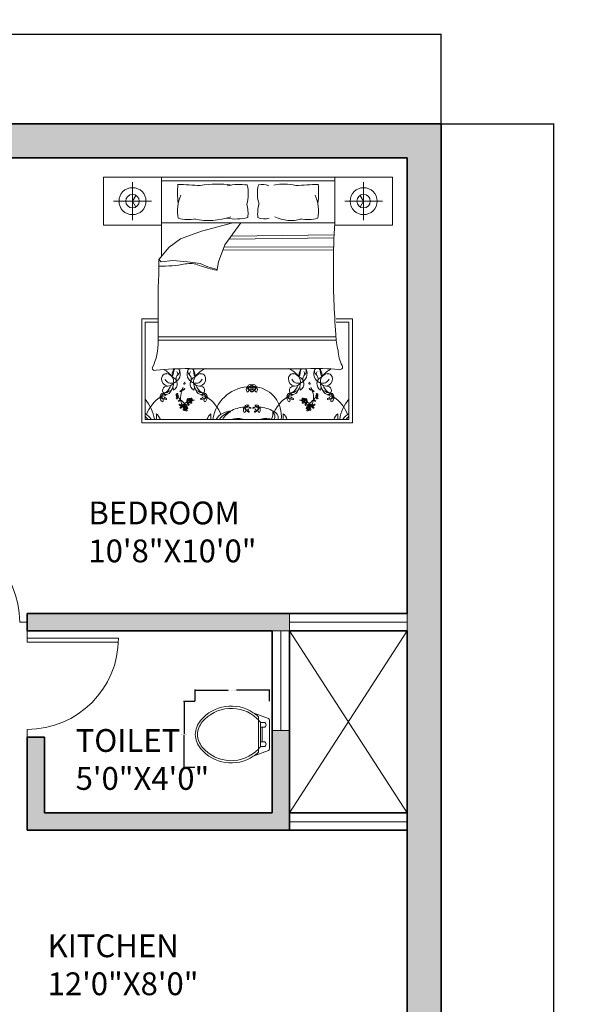
# Model space of a CAD drawing. Units: inches. Extents: x -5 to 366, y -496 to 54.
# Tile 10 of 10: x 214 to 366, y -205 to 54. Entities that reach past the tile are written whole.
import ezdxf

# ---------------------------------------------------------------- set-up
doc = ezdxf.new("R2010")
doc.units = ezdxf.units.IN
doc.header["$MEASUREMENT"] = 0
for name, color, linetype, lineweight in [('A-ANNO-DIMS', 2, 'Continuous', 18), ('A-AREA-IDEN', 7, 'Continuous', 25), ('A-DOOR', 3, 'Continuous', 18), ('A-FLOR-FIXT', 9, 'Continuous', 18), ('A-FLOR-OPEN', 8, 'Continuous', 13), ('A-FURN', 8, 'Continuous', 18), ('A-GLAZ', 4, 'Continuous', 18), ('A-WALL', 7, 'Continuous', 35), ('A-WALL-PATT', 252, 'Continuous', 13)]:
    doc.layers.add(name, color=color, linetype=linetype, lineweight=lineweight)
doc.styles.get("Standard").update_dxf_attribs({"font": 'arial.ttf'})
doc.dimstyles.get("Standard").update_dxf_attribs({"dimtxt": 0.18, "dimasz": 0.18, "dimexe": 0.18, "dimexo": 0.0625, "dimgap": 0.09, "dimtad": 0, "dimtih": 1, "dimtoh": 1, "dimdec": 0, "dimzin": 0, "dimdsep": 46, "dimlunit": 3, "dimtxsty": 'Standard', "dimcen": 0.09, "dimadec": 0, "dimazin": 0, "dimtfac": 1, "dimtdec": 0, "dimtofl": 0, "dimtmove": 0, "dimatfit": 3, "dimfxl": 1, "dimtolj": 1, "dimtzin": 0, "dimarcsym": 0})

# ---------------------------------------------------------------- blocks, each defined once
blk = doc.blocks.new('*D2')
at = {"layer": 'A-ANNO-DIMS', "color": 0, "lineweight": -2, "transparency": 16777216}
for p, q in [((21.93, 26.58), (21.93, 50.16)), ((22.11, 49.98), (162.99, 49.98)), ((324.75, 49.98), (183.88, 49.98)), ((324.93, 26.58), (324.93, 50.16))]:
    blk.add_line(p, q, dxfattribs=at)
at = {"layer": 'A-ANNO-DIMS', "color": 0, "transparency": 16777216}
for points in [[(22.11, 50.01), (22.11, 49.95), (21.93, 49.98)], [(324.75, 50.01), (324.75, 49.95), (324.93, 49.98)]]:
    blk.add_solid(points, dxfattribs=at)
at = {"layer": 'Defpoints', "color": 0, "transparency": 16777216}
for p in [(324.93, 49.98), (21.93, 26.52), (324.93, 26.52)]:
    blk.add_point(p, dxfattribs=at)
at = {"layer": 'A-ANNO-DIMS', "color": 0, "transparency": 16777216, "insert": (173.43, 49.98), "char_height": 6, "attachment_point": 5}
blk.add_mtext('\\A1;25\'-3"', dxfattribs=at)
blk = doc.blocks.new('*D3')
at = {"layer": 'A-ANNO-DIMS', "color": 0, "lineweight": -2, "transparency": 16777216}
for p, q in [((325, 26.52), (354.61, 26.52)), ((354.43, 26.34), (354.43, -212.08)), ((354.43, -456.8), (354.43, -218.38)), ((325, -456.98), (354.61, -456.98))]:
    blk.add_line(p, q, dxfattribs=at)
at = {"layer": 'A-ANNO-DIMS', "color": 0, "transparency": 16777216}
for points in [[(354.4, 26.34), (354.46, 26.34), (354.43, 26.52)], [(354.4, -456.8), (354.46, -456.8), (354.43, -456.98)]]:
    blk.add_solid(points, dxfattribs=at)
at = {"layer": 'Defpoints', "color": 0, "transparency": 16777216}
for p in [(324.93, 26.52), (324.93, -456.98), (354.43, -456.98)]:
    blk.add_point(p, dxfattribs=at)
at = {"layer": 'A-ANNO-DIMS', "color": 0, "transparency": 16777216, "insert": (354.43, -215.23), "char_height": 6, "attachment_point": 5}
blk.add_mtext('\\A1;40\'-4"', dxfattribs=at)
blk = doc.blocks.new('DOOR-SWING-24IN')
for p, q in [((-1, 0), (-1, 24)), ((0, 0), (0, 24))]:
    blk.add_line(p, q)
blk.add_arc((0, 0), 24, 90, 180)
blk = doc.blocks.new('BED-DOUBLE-WITH-NIGHTSTANDS')
for p, q in [((0, 64.67), (76.05, 64.67)), ((7.61, 53.37), (7.61, 63.31)), ((15.21, 64.67), (15.21, 43.8)), ((60.84, 63.7), (15.21, 63.7)), ((68.45, 53.37), (68.45, 63.31)), ((12.58, 58.34), (2.64, 58.34)), ((63.48, 58.34), (73.42, 58.34)), ((15.21, 52.66), (60.84, 52.66)), ((25.78, 50.4), (34.07, 52.66)), ((36.11, 52.66), (31.94, 46.86)), ((20.23, 48.39), (25.78, 50.4)), ((60.64, 49.5), (33.56, 49.12)), ((17.3, 46.24), (20.23, 48.39)), ((31.94, 46.86), (30.24, 42.39)), ((60.61, 48.72), (33, 48.33)), ((14.53, 43.01), (17.3, 46.24)), ((60.58, 45.54), (31.39, 45.42)), ((60.57, 46.32), (31.69, 46.21)), ((15.15, 42.39), (14.53, 43.01)), ((18.23, 42.7), (15.15, 42.39)), ((22.08, 42.39), (18.23, 42.7)), ((25.47, 41.93), (22.08, 42.39)), ((27.47, 41.01), (25.47, 41.93)), ((30.24, 42.39), (29.94, 40.39)), ((29.94, 40.39), (27.47, 41.01)), ((10.04, 27.39), (14.34, 27.39)), ((10.04, 0), (10.04, 27.39)), ((14.34, 26.51), (10.92, 26.51)), ((10.92, 26.51), (10.92, 0.88)), ((64.6, 26.51), (61.25, 26.51)), ((61.27, 27.39), (65.49, 27.39)), ((64.6, 0.88), (64.6, 26.51)), ((65.49, 27.39), (65.49, 0)), ((61.19, 22.65), (14.34, 22.65)), ((61.26, 21.7), (14.34, 21.7)), ((53.47, 14.23), (22.59, 14.23)), ((18.42, 8.59), (18.25, 9.45)), ((23.73, 8.59), (23.9, 9.45)), ((51.79, 8.59), (51.63, 9.45)), ((57.11, 8.59), (57.28, 9.45)), ((10.92, 0.88), (64.6, 0.88)), ((65.49, 0), (10.04, 0))]:
    blk.add_line(p, q)
for points in [[(15.21, 52), (0, 52), (0, 64.67)], [(60.84, 64.67), (60.84, 52), (76.05, 52), (76.05, 64.67)], [(7.61, 58.34), (8.49, 59.87)], [(68.45, 58.34), (67.56, 59.87)], [(7.61, 58.34), (8.49, 56.8)], [(68.45, 58.34), (67.56, 56.8)]]:
    blk.add_lwpolyline(points)
for points in [[(19.58, 62.78, 0.074897), (19.67, 57.81, -0.472817)], [(37.67, 57.53, 0.14099), (37.82, 62.6, 0.235245)], [(40.92, 57.53, -0.14099), (40.77, 62.6, -0.235245)], [(56.48, 62.78, -0.074897), (56.38, 57.81, 0.472817)], [(14.37, 36.04, 0.001242), (14.34, 21.61, -0.127202), (12.81, 14.42)], [(61.17, 23.25, 0.056112), (61.72, 19.07, 0.095341), (62.79, 15.03)]]:
    blk.add_lwpolyline(points, format="xyb")
for centre, radius in [((7.61, 58.34), 3.55), ((7.61, 58.34), 1.77), ((68.45, 58.34), 3.55), ((68.45, 58.34), 1.77), ((22.81, 5.83), 0.194), ((52.72, 5.83), 0.194), ((21.54, 3.79), 0.194), ((53.98, 3.79), 0.194)]:
    blk.add_circle(centre, radius)
for centre, radius, start, end in [((61.5, 786.54), 724.98, 266.68521, 267.14978), ((30, 35.26), 27.58, 82.2196, 99.497), ((35.83, 49.2), 13.55, 81.5249, 103.96), ((41.81, 58.99), 3.76, 63.3437, 106.1026), ((47.45, 49.47), 13.37, 76.3427, 101.1841), ((14.56, 786.54), 724.98, 272.85022, 273.31479), ((29.27, 55.82), 9.8, 155.1316, 191.7583), ((46.79, 55.82), 9.8, 348.2417, 24.8684), ((28.71, 54.99), 9.32, 354.0129, 15.8293), ((49.88, 54.99), 9.32, 164.1707, 185.9871), ((22.29, 63.67), 10.19, 255.1039, 281.0369), ((27.66, 70.91), 17.68, 258.0397, 289.2615), ((34.82, 67.05), 13.41, 259.8617, 283.6238), ((42.32, 57.67), 4.03, 245.0183, 288.5407), ((49.36, 62.92), 9.68, 243.8761, 286.1746), ((53.76, 63.67), 10.19, 258.9631, 284.8961), ((197.18, 43.36), 136.65, 176.1, 180.9282), ((-55.2, 41.12), 69.76, 355.8294, 1.553), ((15.83, 69.94), 28.7, 267.4519, 281.3392), ((22.69, 35.73), 6.19, 66.2616, 101.3392), ((35.22, 69.13), 29.49, 250.1194, 259.3383), ((29.76, 40.33), 0.184, 268.8623, 19.7536), ((238.78, 38.39), 178.26, 179.1145, 184.8735), ((13.51, 14.47), 0.702, 183.98, 297.3412), ((21.68, -64.93), 79.17, 89.3433, 95.6887), ((13.22, 8.88), 5.76, 33.6671, 63.2997), ((20.93, 12.3), 2.93, 145.785, 184.7304), ((15.33, 13.67), 3.15, 328.8218, 9.1554), ((19.23, 13.39), 0.916, 120.0293, 142.325), ((17.77, 12.85), 2.42, 289.2822, 29.1751), ((17.4, 12.41), 2.19, 7.436, 29.9149), ((18.84, 13.57), 1.14, 311.5653, 23.8354), ((19.23, 13.39), 0.916, 44.4517, 63.558), ((24.38, 12.85), 2.42, 150.8249, 250.7178), ((23.31, 13.57), 1.14, 156.1646, 228.4347), ((22.92, 13.39), 0.916, 113.229, 135.5483), ((24.75, 12.41), 2.19, 150.0851, 172.564), ((22.92, 13.39), 0.916, 37.675, 66.7144), ((21.22, 12.3), 2.93, 355.2696, 34.215), ((26.82, 13.67), 3.15, 169.7133, 211.1782), ((28.93, 8.88), 5.76, 111.4941, 146.3329), ((46.59, 8.88), 5.76, 33.6671, 68.5059), ((54.31, 12.3), 2.93, 145.785, 184.7304), ((48.7, 13.67), 3.15, 328.8218, 10.2867), ((52.61, 13.39), 0.916, 113.2856, 142.325), ((51.15, 12.85), 2.42, 289.2822, 29.1751), ((50.78, 12.41), 2.19, 7.436, 29.9149), ((52.61, 13.39), 0.916, 44.4517, 66.7144), ((52.22, 13.57), 1.14, 311.5653, 23.8354), ((55.8, -59.74), 74, 85.2402, 91.8035), ((57.76, 12.85), 2.42, 150.8249, 250.7178), ((56.68, 13.57), 1.14, 156.1646, 228.4347), ((56.3, 13.39), 0.916, 106.6343, 135.5483), ((58.13, 12.41), 2.19, 150.0851, 172.564), ((56.3, 13.39), 0.916, 37.675, 72.5814), ((54.6, 12.3), 2.93, 355.2696, 34.215), ((60.2, 13.67), 3.15, 169.249, 211.1782), ((62.31, 8.88), 5.76, 113.6453, 146.3329), ((62.21, 14.65), 0.693, 246.5219, 33.8264), ((16.57, 11.64), 1.28, 84.4856, 181.0538), ((17.09, 11.46), 1.82, 174.9449, 262.8857), ((17.81, 12.15), 1.76, 201.5819, 291.4221), ((16.17, 10.69), 2.29, 355.2933, 76.921), ((16.78, 11.86), 2.21, 272.3591, 324.0401), ((14.38, 10.75), 4.08, 326.2883, 356.5076), ((17.47, 10.23), 1.89, 299.9085, 73.1337), ((20.93, 12.3), 2.93, 212.7011, 216.3445), ((18.67, 11.02), 0.472, 257.3041, 15.1471), ((20.63, 11.55), 1.56, 131.5653, 195.1471), ((21.29, 10.31), 0.147, 102.7051, 280.4384), ((21.28, 10.4), 0.238, 280.4384, 100.4136), ((21.52, 11.55), 1.56, 344.8529, 48.4347), ((24.67, 10.23), 1.89, 106.8663, 240.0915), ((23.48, 11.02), 0.472, 164.8529, 282.6959), ((21.22, 12.3), 2.93, 323.6555, 327.2989), ((25.37, 11.86), 2.21, 215.9599, 267.6409), ((25.97, 10.69), 2.29, 103.079, 184.7067), ((24.34, 12.15), 1.76, 248.5779, 338.4181), ((27.77, 10.75), 4.08, 183.4924, 213.7117), ((25.05, 11.46), 1.82, 277.1143, 5.0551), ((25.58, 11.64), 1.28, 358.9462, 95.5144), ((49.95, 11.64), 1.28, 84.4856, 181.0538), ((50.47, 11.46), 1.82, 174.9449, 262.8857), ((51.19, 12.15), 1.76, 201.5819, 291.4221), ((49.55, 10.69), 2.29, 355.2933, 76.921), ((50.16, 11.86), 2.21, 272.3591, 324.0401), ((47.76, 10.75), 4.08, 326.2883, 356.5076), ((50.85, 10.23), 1.89, 299.9085, 73.1337), ((54.31, 12.3), 2.93, 212.7011, 216.3445), ((52.05, 11.02), 0.472, 257.3041, 15.1471), ((54.01, 11.55), 1.56, 131.5653, 195.1471), ((54.25, 10.4), 0.238, 79.5864, 259.5616), ((54.23, 10.31), 0.147, 259.5616, 77.2949), ((54.89, 11.55), 1.56, 344.8529, 48.4347), ((58.05, 10.23), 1.89, 106.8663, 240.0915), ((56.86, 11.02), 0.472, 164.8529, 282.6959), ((54.6, 12.3), 2.93, 323.6555, 327.2989), ((58.75, 11.86), 2.21, 215.9599, 267.6409), ((59.35, 10.69), 2.29, 103.079, 184.7067), ((57.72, 12.15), 1.76, 248.5779, 338.4181), ((61.15, 10.75), 4.08, 183.4924, 213.7117), ((58.43, 11.46), 1.82, 277.1143, 5.0551), ((58.96, 11.64), 1.28, 358.9462, 95.5144), ((16.68, 8.53), 1.14, 80.264, 250.8688), ((16.44, 7.29), 0.7, 63.9755, 143.2681), ((14.41, 11.04), 3.59, 301.2614, 341.7045), ((16.4, 8.87), 1.43, 265.969, 344.3045), ((17.94, 6.98), 1.52, 96.1662, 141.5825), ((20.45, 8.04), 0.399, 101.3256, 154.4621), ((19.88, 9.4), 1.2, 280.2588, 300.656), ((20.15, 10.36), 2.14, 268.3264, 277.1302), ((26.56, 6.48), 6.3, 163.5842, 183.8277), ((19.62, 9.39), 1.22, 308.2101, 316.3071), ((20.37, 8.59), 0.365, 278.3432, 4.2869), ((20.17, 8.91), 0.637, 300.656, 332.6341), ((20.64, 8.49), 0.155, 55.7657, 157.4417), ((26.56, 6.48), 6.3, 153.0032, 159.8941), ((20.89, 8.63), 0.155, 84.3784, 186.0543), ((20.74, 9.25), 0.637, 269.1859, 301.164), ((20.93, 8.93), 0.365, 237.5332, 323.4768), ((20.57, 9.97), 1.22, 285.5129, 293.6099), ((21.37, 8.59), 0.399, 87.3579, 140.4944), ((20.45, 9.74), 1.2, 301.164, 321.5612), ((19.47, 9.95), 2.14, 324.6898, 333.4936), ((27.73, 11.04), 3.59, 198.2955, 238.7386), ((24.21, 6.98), 1.52, 38.4175, 83.8338), ((25.74, 8.87), 1.43, 195.6955, 274.031), ((25.47, 8.53), 1.14, 289.1312, 99.736), ((25.71, 7.29), 0.7, 36.7319, 116.0245), ((38.62, -0.46), 9.93, 94.4623, 172.255), ((38.66, 8.7), 1.1, 137.7873, 219.1145), ((37.41, 8.74), 0.829, 298.5391, 58.3627), ((38.64, 9.21), 0.823, 63.0274, 163.8037), ((37.8, 11.14), 1.7, 271.4585, 315.3727), ((38.49, 8.01), 1.57, 45.5411, 114.3101), ((39.93, 16.07), 6.95, 252.593, 267.2582), ((38.66, 9.41), 0.812, 177.7585, 283.852), ((40.22, 10.26), 2.51, 198.9159, 238.011), ((39.57, 8.01), 1.57, 65.6899, 134.4589), ((38.14, 16.07), 6.95, 272.7418, 287.407), ((38.83, 8.73), 0.107, 283.852, 219.9245), ((38.96, 8.23), 0.123, 238.011, 71.5592), ((38.98, 8.29), 0.0599, 71.5592, 188.0167), ((39.1, 8.23), 0.123, 108.4408, 301.989), ((39.42, 9.21), 0.823, 16.1963, 116.9726), ((40.26, 11.14), 1.7, 224.6273, 268.5415), ((39.08, 8.29), 0.0599, 351.9833, 108.4408), ((39.22, 8.77), 0.0647, 320.1909, 256.0209), ((37.84, 10.26), 2.51, 301.989, 341.0841), ((39.4, 9.41), 0.812, 256.148, 2.2415), ((40.65, 8.74), 0.829, 121.6373, 241.4609), ((39.4, 8.7), 1.1, 320.8855, 42.2127), ((39.12, 1.83), 7.69, 352.8636, 81.8197), ((50.06, 8.53), 1.14, 80.264, 250.8688), ((49.82, 7.29), 0.7, 63.9755, 143.2681), ((47.79, 11.04), 3.59, 301.2614, 341.7045), ((49.78, 8.87), 1.43, 265.969, 344.3045), ((51.32, 6.98), 1.52, 96.1662, 141.5825), ((55.08, 9.74), 1.2, 218.4388, 238.836), ((54.15, 8.59), 0.399, 39.5056, 92.6421), ((56.06, 9.95), 2.14, 206.5064, 215.3102), ((54.6, 8.93), 0.365, 216.5232, 302.4668), ((54.95, 9.97), 1.22, 246.3901, 254.4871), ((54.79, 9.25), 0.637, 238.836, 270.8141), ((48.96, 6.48), 6.3, 20.1059, 26.9968), ((54.64, 8.63), 0.155, 353.9457, 95.6216), ((54.88, 8.49), 0.155, 22.5583, 124.2343), ((55.16, 8.59), 0.365, 175.7131, 261.6568), ((55.36, 8.91), 0.637, 207.3659, 239.344), ((48.96, 6.48), 6.3, 356.1723, 16.4158), ((55.91, 9.39), 1.22, 223.6929, 231.7899), ((55.65, 9.4), 1.2, 239.344, 259.7412), ((55.37, 10.36), 2.14, 262.8698, 271.6736), ((55.07, 8.04), 0.399, 25.5379, 78.6744), ((61.11, 11.04), 3.59, 198.2955, 238.7386), ((59.12, 8.87), 1.43, 195.6955, 274.031), ((57.59, 6.98), 1.52, 38.4175, 83.8338), ((58.85, 8.53), 1.14, 289.1312, 99.736), ((59.08, 7.29), 0.7, 36.7319, 116.0245), ((3.53, -0.46), 9.93, 7.745, 41.8856), ((20.52, -1.44), 9.93, 124.3865, 158.5908), ((15.99, 6.52), 1.1, 167.7115, 249.0387), ((15.71, 6.95), 0.823, 92.9516, 193.728), ((14.03, 8.2), 1.7, 301.3827, 345.2969), ((16.18, 5.84), 1.57, 75.4653, 144.2343), ((13.4, 13.54), 6.95, 282.5173, 297.1824), ((14.89, 5.93), 0.829, 328.4633, 88.2869), ((16.56, 8.65), 2.51, 228.8402, 267.9352), ((15.63, 7.13), 0.812, 207.6827, 313.7762), ((16.12, 6.62), 0.107, 313.7762, 249.7183), ((16.46, 6.32), 0.0599, 101.4834, 217.9409), ((16.48, 6.26), 0.123, 267.9352, 101.4834), ((19.32, 7.28), 0.323, 101.5637, 142.6358), ((19.06, 6.98), 0.194, 273.2768, 86.7232), ((19.32, 6.63), 0.32, 217.7621, 259.0403), ((19.28, 7.17), 0.185, 91.1081, 181.8675), ((19.66, 7.05), 0.588, 203.4276, 227.6104), ((19.48, 6.8), 0.4, 80.3487, 133.6538), ((19.41, 7.13), 0.317, 229.7889, 317.6792), ((19.06, 7.54), 0.466, 288.7263, 352.5032), ((19.05, 6.46), 0.45, 355.053, 68.3618), ((19.4, 6.38), 0.634, 83.0852, 105.7171), ((19.38, 7.52), 0.15, 345.2356, 144.9248), ((19.35, 6.43), 0.149, 232.4737, 355.053), ((15.01, 1.12), 7.22, 43.1541, 52.0459), ((19.52, 7.03), 0.167, 317.6792, 80.3487), ((20, 5.48), 0.399, 101.3256, 154.4621), ((19.42, 6.84), 1.2, 280.2588, 300.656), ((19.7, 7.8), 2.14, 268.3264, 277.1302), ((19.17, 6.83), 1.22, 308.2101, 316.3071), ((19.91, 6.03), 0.365, 278.3432, 4.2869), ((19.71, 6.35), 0.637, 300.656, 332.6341), ((20.19, 5.93), 0.155, 55.7657, 157.4417), ((23.43, 6.32), 3.16, 184.756, 209.2041), ((27.97, 13.04), 10.39, 222.2412, 232.1744), ((23.75, 2.13), 3.79, 120.544, 139.818), ((21.33, 6.12), 0.883, 304.5369, 16.3699), ((21.8, 5.92), 0.537, 272.8499, 356.1226), ((21.42, 5.72), 0.52, 321.7607, 7.9252), ((21.53, 4.97), 0.52, 8.7227, 54.8872), ((21.56, 4.55), 0.883, 0.278, 72.111), ((22.55, 5.87), 0.625, 127.3105, 187.9252), ((21.95, 4.88), 0.537, 20.5253, 88.5375), ((21.7, 5.94), 0.641, 355.0106, 41.658), ((22.4, 5.47), 0.192, 148.0499, 225.6268), ((23.75, 2.13), 3.79, 113.0501, 113.8477), ((22.76, 5.25), 0.611, 104.7558, 148.0499), ((22.42, 5.69), 0.382, 247.4086, 351.4386), ((22.6, 6.1), 0.264, 126.1046, 271.4281), ((22.57, 6.17), 0.19, 353.7526, 131.7054), ((22.52, 5.67), 0.128, 262.906, 7.132), ((22.39, 5.95), 0.267, 0.0645, 61.1507), ((22.45, 6.18), 0.305, 311.8413, 355.7877), ((23.07, 5.47), 0.32, 151.2196, 259.0403), ((23.08, 6.13), 0.323, 101.5637, 176.365), ((23.04, 6.02), 0.185, 91.1081, 181.8675), ((23.42, 5.9), 0.588, 203.4276, 227.6104), ((23.23, 5.64), 0.4, 80.3487, 133.6538), ((23.16, 5.98), 0.317, 229.7889, 317.6792), ((22.82, 6.39), 0.466, 288.7263, 352.5032), ((22.8, 5.3), 0.45, 355.053, 68.3618), ((23.16, 5.23), 0.634, 83.0852, 105.7171), ((23.14, 6.36), 0.15, 345.2356, 144.9248), ((23.1, 5.28), 0.149, 232.4737, 355.053), ((23.27, 5.87), 0.167, 317.6792, 80.3487), ((23.75, 2.13), 3.79, 87.1071, 94.7585), ((25.67, 6.26), 0.123, 78.5166, 272.0648), ((25.96, 5.84), 1.57, 35.7657, 104.5347), ((28.74, 13.54), 6.95, 242.8176, 257.4827), ((25.58, 8.65), 2.51, 272.0648, 311.1598), ((25.68, 6.32), 0.0599, 322.0591, 78.5166), ((26.52, 7.13), 0.812, 226.2238, 332.3173), ((26.04, 6.66), 0.0647, 290.2667, 226.2271), ((27.26, 5.93), 0.829, 91.7131, 211.5367), ((26.44, 6.95), 0.823, 346.272, 87.0484), ((28.12, 8.2), 1.7, 194.7031, 238.6173), ((26.16, 6.52), 1.1, 290.9613, 12.2885), ((21.63, -1.44), 9.93, 21.4092, 55.6135), ((53.9, -1.44), 9.93, 124.3865, 158.5908), ((49.36, 6.52), 1.1, 167.7115, 249.0387), ((49.09, 6.95), 0.823, 92.9516, 193.728), ((47.41, 8.2), 1.7, 301.3827, 345.2969), ((49.56, 5.84), 1.57, 75.4653, 144.2343), ((46.78, 13.54), 6.95, 282.5173, 297.1824), ((49.01, 7.13), 0.812, 207.6827, 313.7762), ((49.94, 8.65), 2.51, 228.8402, 267.9352), ((48.26, 5.93), 0.829, 328.4633, 88.2869), ((49.5, 6.62), 0.107, 313.7762, 249.7183), ((49.84, 6.32), 0.0599, 101.4834, 217.9409), ((49.86, 6.26), 0.123, 267.9352, 101.4834), ((51.78, 2.13), 3.79, 85.2415, 92.8929), ((52.25, 5.87), 0.167, 99.6513, 222.3208), ((52.37, 5.98), 0.317, 222.3208, 310.2111), ((52.29, 5.64), 0.4, 46.3462, 99.6513), ((52.39, 6.36), 0.15, 35.0752, 194.7644), ((52.71, 6.39), 0.466, 187.4968, 251.2737), ((52.72, 5.3), 0.45, 111.6382, 184.947), ((52.42, 5.28), 0.149, 184.947, 307.5263), ((52.37, 5.23), 0.634, 74.2829, 96.9148), ((52.49, 6.02), 0.185, 358.1325, 88.8919), ((52.11, 5.9), 0.588, 312.3896, 336.5724), ((52.45, 6.13), 0.323, 3.635, 78.4363), ((52.45, 5.47), 0.32, 280.9597, 28.7804), ((53.11, 5.69), 0.382, 188.5614, 292.5914), ((52.96, 6.17), 0.19, 48.2946, 186.2474), ((53.07, 6.18), 0.305, 184.2123, 228.1587), ((53.14, 5.95), 0.267, 118.8493, 179.9355), ((53, 5.67), 0.128, 172.868, 277.094), ((52.93, 6.1), 0.264, 268.5719, 53.8954), ((52.77, 5.25), 0.611, 31.9501, 75.2442), ((53.57, 4.88), 0.537, 91.4625, 159.4747), ((53.97, 4.55), 0.883, 107.889, 179.722), ((53.83, 5.94), 0.641, 138.342, 184.9894), ((53.73, 5.92), 0.537, 183.8774, 267.1501), ((51.78, 2.13), 3.79, 66.1523, 66.9499), ((53.12, 5.47), 0.192, 314.3732, 31.9501), ((54.2, 6.12), 0.883, 163.6301, 235.4631), ((52.97, 5.87), 0.625, 352.0748, 52.6895), ((54, 4.97), 0.52, 125.1128, 171.2773), ((54.11, 5.72), 0.52, 172.0748, 218.2393), ((51.78, 2.13), 3.79, 40.182, 59.456), ((47.55, 13.04), 10.39, 307.8256, 317.7588), ((52.1, 6.32), 3.16, 330.7959, 355.244), ((60.52, 1.12), 7.22, 127.9541, 136.8459), ((55.33, 5.93), 0.155, 22.5583, 124.2343), ((55.61, 6.03), 0.365, 175.7131, 261.6568), ((55.81, 6.35), 0.637, 207.3659, 239.344), ((56.36, 6.83), 1.22, 223.6929, 231.7899), ((56.1, 6.84), 1.2, 239.344, 259.7412), ((55.82, 7.8), 2.14, 262.8698, 271.6736), ((55.53, 5.48), 0.399, 25.5379, 78.6744), ((56.01, 7.03), 0.167, 99.6513, 222.3208), ((56.12, 7.13), 0.317, 222.3208, 310.2111), ((56.05, 6.8), 0.4, 46.3462, 99.6513), ((56.15, 7.52), 0.15, 35.0752, 194.7644), ((56.46, 7.54), 0.466, 187.4968, 251.2737), ((56.48, 6.46), 0.45, 111.6382, 184.947), ((56.18, 6.43), 0.149, 184.947, 307.5263), ((56.12, 6.38), 0.634, 74.2829, 96.9148), ((56.25, 7.17), 0.185, 358.1325, 88.8919), ((55.86, 7.05), 0.588, 312.3896, 336.5724), ((56.2, 7.28), 0.323, 37.3642, 78.4363), ((56.21, 6.63), 0.32, 280.9597, 322.2379), ((56.47, 6.98), 0.194, 93.2768, 266.7232), ((59.05, 6.26), 0.123, 78.5166, 272.0648), ((59.34, 5.84), 1.57, 35.7657, 104.5347), ((62.12, 13.54), 6.95, 242.8176, 257.4827), ((58.96, 8.65), 2.51, 272.0648, 311.1598), ((59.06, 6.32), 0.0599, 322.0591, 78.5166), ((59.9, 7.13), 0.812, 226.2238, 332.3173), ((59.42, 6.66), 0.0647, 290.2667, 226.2271), ((60.64, 5.93), 0.829, 91.7131, 211.5367), ((61.5, 8.2), 1.7, 194.7031, 238.6173), ((59.82, 6.95), 0.823, 346.272, 87.0484), ((59.54, 6.52), 1.1, 290.9613, 12.2885), ((55.01, -1.44), 9.93, 21.4092, 55.6135), ((72, -0.46), 9.93, 138.1144, 172.255), ((20.13, 4.78), 0.216, 146.8636, 236.9021), ((23.18, 9.55), 5.66, 235.1882, 238.8844), ((20.5, 5.1), 0.585, 199.4799, 267.6828), ((20.44, 4.87), 0.504, 212.8155, 277.3992), ((20.15, 4.54), 0.585, 266.9701, 338.2913), ((17.06, 8.72), 5.66, 302.6784, 306.3746), ((20.29, 4.07), 0.216, 214.3538, 304.3923), ((20.37, 4.89), 0.224, 238.8844, 314.2646), ((20.33, 4.39), 0.504, 280.3057, 17.1958), ((20.28, 4.34), 0.224, 306.3746, 21.7548), ((20.65, 4.49), 0.169, 19.3605, 201.7548), ((20.65, 4.61), 0.169, 311.8703, 134.2646), ((23.82, 3.07), 3.37, 153.7819, 158.2913), ((21.14, 5.38), 0.883, 247.2305, 319.0635), ((20.85, 5.08), 0.52, 264.4544, 310.6188), ((23.43, 6.32), 3.16, 214.0033, 222.4917), ((21.23, 4.87), 0.537, 218.3208, 298.8162), ((21.14, 3.43), 0.192, 148.0499, 225.6268), ((21.49, 3.21), 0.611, 104.7558, 148.0499), ((21.15, 3.64), 0.382, 247.4086, 351.4386), ((21.33, 4.06), 0.264, 126.1046, 271.4281), ((21.3, 4.13), 0.19, 353.7526, 131.7054), ((21.59, 4.21), 0.625, 70.0041, 130.6188), ((21.26, 3.63), 0.128, 262.906, 7.132), ((21.12, 3.91), 0.267, 0.0645, 61.1507), ((21.18, 4.13), 0.305, 311.8413, 355.7877), ((21.19, 4.97), 0.641, 297.7043, 344.3516), ((21.81, 4.09), 0.323, 101.5637, 176.365), ((21.81, 3.43), 0.32, 151.2196, 259.0403), ((21.77, 3.98), 0.185, 91.1081, 181.8675), ((22.15, 3.86), 0.588, 203.4276, 227.6104), ((21.97, 3.6), 0.4, 80.3487, 133.6538), ((21.89, 3.93), 0.317, 229.7889, 317.6792), ((21.55, 4.35), 0.466, 288.7263, 352.5032), ((21.54, 3.26), 0.45, 355.053, 68.3618), ((21.89, 3.19), 0.634, 83.0852, 105.7171), ((21.87, 4.32), 0.15, 345.2356, 144.9248), ((21.84, 3.24), 0.149, 232.4737, 355.053), ((22, 3.83), 0.167, 317.6792, 80.3487), ((22.66, 5.14), 0.625, 188.7227, 249.3375), ((21.86, 4.83), 0.641, 334.9899, 21.6373), ((33.64, -1.79), 4.84, 91.272, 146.5383), ((35.38, -2.69), 6.03, 107.8504, 143.6964), ((38.55, -4.39), 8.97, 124.0123, 144.053), ((37.86, -5.78), 9.93, 94.4623, 117.4146), ((37.9, 3.38), 1.1, 137.7873, 219.1145), ((36.65, 3.42), 0.829, 298.5391, 58.3627), ((37.88, 3.89), 0.823, 63.0274, 163.8037), ((37.04, 5.82), 1.7, 271.4585, 315.3727), ((37.73, 2.69), 1.57, 45.5411, 114.3101), ((39.46, 4.94), 2.51, 198.9159, 238.011), ((39.17, 10.75), 6.95, 252.593, 267.2582), ((37.9, 4.09), 0.812, 177.7585, 283.852), ((38.07, 3.41), 0.107, 283.852, 219.9245), ((38.2, 2.91), 0.123, 238.011, 71.5592), ((38.22, 2.97), 0.0599, 71.5592, 188.0167), ((40.33, 2.69), 1.57, 65.6899, 134.4589), ((38.9, 10.75), 6.95, 272.7418, 287.407), ((39.86, 2.91), 0.123, 108.4408, 301.989), ((40.18, 3.89), 0.823, 16.1963, 116.9726), ((41.02, 5.82), 1.7, 224.6273, 268.5415), ((39.84, 2.97), 0.0599, 351.9833, 108.4408), ((39.98, 3.45), 0.0647, 320.1909, 256.0209), ((38.6, 4.94), 2.51, 301.989, 341.0841), ((40.16, 4.09), 0.812, 256.148, 2.2415), ((41.41, 3.42), 0.829, 121.6373, 241.4609), ((40.16, 3.38), 1.1, 320.8855, 42.2127), ((40.2, -5.78), 9.93, 62.5854, 85.5377), ((40.11, 2.54), 4.45, 338.117, 6.6195), ((44.19, 1.3), 1.78, 346.3898, 79.0739), ((42.85, 1.54), 2.25, 342.8609, 41.9049), ((53.67, 4.83), 0.641, 158.3627, 205.0101), ((52.87, 5.14), 0.625, 290.6625, 351.2773), ((53.52, 3.83), 0.167, 99.6513, 222.3208), ((53.63, 3.93), 0.317, 222.3208, 310.2111), ((53.56, 3.6), 0.4, 46.3462, 99.6513), ((53.66, 4.32), 0.15, 35.0752, 194.7644), ((53.97, 4.35), 0.466, 187.4968, 251.2737), ((53.99, 3.26), 0.45, 111.6382, 184.947), ((53.69, 3.24), 0.149, 184.947, 307.5263), ((53.64, 3.19), 0.634, 74.2829, 96.9148), ((53.93, 4.21), 0.625, 49.3812, 109.9959), ((54.39, 5.38), 0.883, 220.9365, 292.7695), ((54.34, 4.97), 0.641, 195.6484, 242.2957), ((53.76, 3.98), 0.185, 358.1325, 88.8919), ((53.37, 3.86), 0.588, 312.3896, 336.5724), ((53.72, 4.09), 0.323, 3.635, 78.4363), ((53.72, 3.43), 0.32, 280.9597, 28.7804), ((54.38, 3.64), 0.382, 188.5614, 292.5914), ((54.3, 4.87), 0.537, 241.1838, 321.6792), ((54.23, 4.13), 0.19, 48.2946, 186.2474), ((54.34, 4.13), 0.305, 184.2123, 228.1587), ((54.4, 3.91), 0.267, 118.8493, 179.9355), ((54.27, 3.63), 0.128, 172.868, 277.094), ((54.2, 4.06), 0.264, 268.5719, 53.8954), ((54.03, 3.21), 0.611, 31.9501, 75.2442), ((54.68, 5.08), 0.52, 229.3812, 275.5456), ((52.1, 6.32), 3.16, 317.5083, 325.9967), ((54.39, 3.43), 0.192, 314.3732, 31.9501), ((55.2, 4.39), 0.504, 162.8042, 259.6943), ((54.88, 4.61), 0.169, 45.7354, 228.1297), ((54.88, 4.49), 0.169, 338.2452, 160.6395), ((51.7, 3.07), 3.37, 21.7087, 26.2181), ((55.38, 4.54), 0.585, 201.7087, 273.0299), ((55.15, 4.89), 0.224, 225.7354, 301.1156), ((55.09, 4.87), 0.504, 262.6008, 327.1845), ((55.24, 4.34), 0.224, 158.2452, 233.6254), ((55.02, 5.1), 0.585, 272.3172, 340.5201), ((58.47, 8.72), 5.66, 233.6254, 237.3216), ((55.23, 4.07), 0.216, 235.6077, 325.6462), ((52.34, 9.55), 5.66, 301.1156, 304.8118), ((55.39, 4.78), 0.216, 303.0979, 33.1364), ((8.51, -1.79), 4.84, 33.4617, 60.1116), ((6.77, -2.69), 6.03, 36.3036, 46.4814), ((11.22, -0.67), 4.04, 22.5547, 48.9546), ((0.16, 1.5), 13.74, 357.4081, 3.6519), ((30.93, -0.67), 4.04, 131.0454, 157.4453), ((41.99, 1.5), 13.74, 176.3481, 182.5919), ((35.08, -4.34), 5.46, 73.5431, 107.0202), ((37.25, -7.16), 8.08, 94.3787, 95.6357), ((41.5, -12.69), 14.43, 109.7217, 109.9028), ((42.98, -4.34), 5.46, 72.9798, 106.4569), ((40.82, -7.16), 8.08, 84.3643, 85.6213), ((36.56, -12.69), 14.43, 70.0972, 70.2783), ((33.54, 1.5), 13.74, 357.4081, 3.6519), ((44.6, -0.67), 4.04, 22.5547, 48.9546), ((64.31, -0.67), 4.04, 131.0454, 157.4453), ((75.37, 1.5), 13.74, 176.3481, 182.5919), ((67.02, -1.79), 4.84, 119.8884, 146.5383), ((68.76, -2.69), 6.03, 133.5186, 143.6964)]:
    blk.add_arc(centre, radius, start, end)
blk = doc.blocks.new('WC-PLAN')
for p, q in [((16.62, 12.16), (16.62, 11.34)), ((16.62, 11.34), (16.62, 7.48)), ((16.62, 3.63), (16.62, 7.48)), ((16.62, 3.63), (16.62, 2.81))]:
    blk.add_line(p, q)
for points in [[(15.28, 13.22, 0.383919), (1.41, 11.17, 0.163732), (0, 7.48, 0.359733)], [(16.22, 11.73, 0.431639), (1.86, 10.79, 0.162618), (0.58, 7.48, 0.470877)], [(16.62, 12.16, 0.040937), (15.28, 13.22, 0.163732)], [(19.59, 7.48), (19.59, 11.23, 0.31031), (19.28, 11.68), (15.28, 13.22, 0.209071)], [(16.62, 11.34, 0.014165), (16.22, 11.73, 0.162618)], [(17.22, 10.66, 0.022712), (16.62, 11.34, 0.162618)], [(17.22, 7.48), (17.22, 10.66, 0.022712)], [(17.22, 10.66), (18.04, 10.66, -1), (18.04, 9.41), (17.61, 9.41)], [(15.28, 1.75, -0.383919), (1.41, 3.8, -0.163732), (0, 7.48, -0.359733)], [(16.62, 3.63, -0.448546), (1.86, 4.17, -0.162618), (0.58, 7.48, -0.470877)], [(19.59, 7.48), (19.59, 3.74, -0.31031), (19.28, 3.28), (15.28, 1.75, -0.209071)], [(17.22, 7.48), (17.22, 4.31, -0.476108)], [(17.22, 4.31), (18.04, 4.31, 1), (18.04, 5.56), (17.61, 5.56)], [(16.62, 2.81, -0.040937), (15.28, 1.75, -0.163732)], [(17.22, 4.31, -0.022712), (16.62, 3.63, -0.162618)]]:
    blk.add_lwpolyline(points, format="xyb")
for points in [[(17.61, 9.41), (17.22, 9.41)], [(17.61, 5.56), (17.61, 9.41)], [(17.61, 5.56), (17.22, 5.56)]]:
    blk.add_lwpolyline(points)
blk = doc.blocks.new('*D19')
at = {"layer": 'A-ANNO-DIMS', "color": 0, "lineweight": -2, "transparency": 16777216}
for p, q in [((260.15, -125.55), (260.15, -122.5)), ((260.33, -122.68), (268.85, -122.68)), ((279.56, -122.68), (271.04, -122.68)), ((279.74, -125.55), (279.74, -122.5))]:
    blk.add_line(p, q, dxfattribs=at)
at = {"layer": 'A-ANNO-DIMS', "color": 0, "transparency": 16777216}
for points in [[(260.33, -122.65), (260.33, -122.71), (260.15, -122.68)], [(279.56, -122.65), (279.56, -122.71), (279.74, -122.68)]]:
    blk.add_solid(points, dxfattribs=at)
at = {"layer": 'Defpoints', "color": 0, "transparency": 16777216}
for p in [(279.74, -122.68), (260.15, -125.62), (279.74, -125.62)]:
    blk.add_point(p, dxfattribs=at)
at = {"layer": 'A-ANNO-DIMS', "color": 0, "transparency": 16777216, "insert": (269.94, -122.68), "char_height": 0.18, "attachment_point": 5}
blk.add_mtext('\\A1;WC 1\'-7 1/2" TYP.', dxfattribs=at)
blk = doc.blocks.new('*D20')
at = {"layer": 'A-ANNO-DIMS', "color": 0, "lineweight": -2, "transparency": 16777216}
for p, q in [((260.08, -125.62), (257.03, -125.62)), ((257.21, -125.8), (257.21, -134.14)), ((257.21, -142.84), (257.21, -134.5)), ((260.08, -143.02), (257.03, -143.02))]:
    blk.add_line(p, q, dxfattribs=at)
at = {"layer": 'A-ANNO-DIMS', "color": 0, "transparency": 16777216}
for points in [[(257.18, -125.8), (257.24, -125.8), (257.21, -125.62)], [(257.18, -142.84), (257.24, -142.84), (257.21, -143.02)]]:
    blk.add_solid(points, dxfattribs=at)
at = {"layer": 'Defpoints', "color": 0, "transparency": 16777216}
for p in [(257.21, -125.62), (260.15, -125.62), (260.15, -143.02)]:
    blk.add_point(p, dxfattribs=at)
at = {"layer": 'A-ANNO-DIMS', "color": 0, "transparency": 16777216, "insert": (257.21, -134.32), "char_height": 0.18, "attachment_point": 5}
blk.add_mtext('\\A1;1\'-5 1/2" TYP.', dxfattribs=at)

msp = doc.modelspace()

# ---------------------------------------------------------------- hatches: boundary and pattern name
at = {"layer": 'A-WALL-PATT'}
h = msp.add_hatch(color=256, dxfattribs=at)
h.dxf.hatch_style = 1
h.paths.add_polyline_path([(324.93, 26.52), (21.93, 26.52), (21.93, -456.98), (26.43, -456.98), (26.43, -331.98), (30.93, -331.98), (30.93, -322.98), (30.93, -106.98), (110.93, -106.98), (110.93, -104.73), (110.93, -102.48), (30.93, -102.48), (30.93, 17.52), (138.93, 17.52), (141.18, 17.52), (143.43, 17.52), (183.43, 17.52), (187.93, 17.52), (315.93, 17.52), (315.93, -102.48), (315.93, -106.98), (315.93, -255.48), (171.93, -255.48), (171.93, -155.84), (167.43, -155.84), (167.43, -291.98), (171.93, -291.98), (171.93, -259.98), (315.93, -259.98), (315.93, -375.98), (297.93, -375.98), (297.93, -380.48), (315.93, -380.48), (315.93, -452.48), (315.93, -456.98), (324.93, -456.98)])
h.paths.add_polyline_path([(143.43, -18.48), (143.43, -13.98), (138.93, -13.98), (138.93, -106.98), (187.93, -106.98), (187.93, -102.48), (143.43, -102.48)], flags=17)
h = msp.add_hatch(color=256, dxfattribs=at)
h.dxf.hatch_style = 1
h.paths.add_polyline_path([(187.93, -13.98), (183.43, -13.98), (163.43, -13.98), (163.43, -18.48), (183.43, -18.48), (183.43, -74.48), (185.68, -74.48), (187.93, -74.48)])
h.paths.add_polyline_path([(284.93, -102.48), (215.93, -102.48), (215.93, -104.73), (215.93, -106.98), (280.43, -106.98), (284.93, -106.98)])
h.paths.add_polyline_path([(284.93, -133.23), (280.43, -133.23), (280.43, -154.98), (220.43, -154.98), (220.43, -134.98), (215.93, -134.98), (215.93, -159.48), (284.93, -159.48)])
h.paths.add_polyline_path([(139.43, -322.98), (123.64, -322.98), (123.64, -331.98), (139.43, -331.98)])
h.paths.add_polyline_path([(171.93, -319.98), (167.43, -319.98), (167.43, -331.98), (171.93, -331.98)])
h.paths.add_polyline_path([(269.93, -375.98), (171.93, -375.98), (167.43, -375.98), (167.43, -380.48), (171.93, -380.48), (265.43, -380.48), (265.43, -452.48), (171.93, -452.48), (167.43, -452.48), (167.43, -456.98), (281.67, -456.98), (281.67, -452.48), (269.93, -452.48), (269.93, -380.48)])

# ---------------------------------------------------------------- linework, layer by layer
at = {"layer": 'A-DOOR'}
for p, q in [((213.93, -104.73), (215.93, -104.73)), ((215.93, -106.98), (215.93, -109.98)), ((215.93, -132.98), (215.93, -134.98))]:
    msp.add_line(p, q, dxfattribs=at)
at = {"layer": 'A-FLOR-OPEN'}
for p, q in [((284.93, -106.98), (315.93, -154.98)), ((315.93, -106.98), (284.93, -154.98))]:
    msp.add_line(p, q, dxfattribs=at)
at = {"layer": 'A-GLAZ'}
for p, q in [((284.93, -106.98), (284.93, -102.48)), ((315.93, -102.48), (315.93, -106.98)), ((315.93, -104.73), (284.93, -104.73)), ((280.43, -106.98), (284.93, -106.98)), ((282.68, -133.23), (282.68, -106.98)), ((284.93, -133.23), (280.43, -133.23)), ((284.93, -157.31), (315.93, -157.31))]:
    msp.add_line(p, q, dxfattribs=at)
at = {"layer": 'A-WALL'}
for p, q in [((21.93, 26.52), (324.93, 26.52)), ((324.93, 26.52), (324.93, -456.98)), ((187.93, 17.52), (315.93, 17.52)), ((315.93, 17.52), (315.93, -102.48)), ((215.93, -102.48), (315.93, -102.48)), ((215.93, -104.73), (215.93, -102.48)), ((215.93, -104.73), (215.93, -106.98)), ((215.93, -106.98), (280.43, -106.98)), ((280.43, -106.98), (280.43, -154.98)), ((284.93, -106.98), (284.93, -159.48)), ((284.93, -106.98), (315.93, -106.98)), ((315.93, -106.98), (315.93, -255.48)), ((215.93, -134.98), (215.93, -159.48)), ((215.93, -134.98), (220.43, -134.98)), ((220.43, -134.98), (220.43, -154.98)), ((220.43, -154.98), (280.43, -154.98)), ((284.93, -154.98), (315.93, -154.98)), ((215.93, -159.48), (315.93, -159.48))]:
    msp.add_line(p, q, dxfattribs=at)

# ---------------------------------------------------------------- block references
at = {"layer": 'A-DOOR', "extrusion": (0, 0, -1), "zscale": -1}
msp.add_blockref('DOOR-SWING-24IN', (-189.93, -104.73), dxfattribs=at)
at = {"layer": 'A-DOOR', "extrusion": (0, 0, -1), "zscale": -1, "rotation": 89.99999999999991}
msp.add_blockref('DOOR-SWING-24IN', (-215.93, -108.98), dxfattribs=at)
at = {"layer": 'A-FLOR-FIXT'}
msp.add_blockref('WC-PLAN', (260.15, -141.8), dxfattribs=at)
at = {"layer": 'A-FURN'}
msp.add_blockref('BED-DOUBLE-WITH-NIGHTSTANDS', (236.02, -52.21), dxfattribs=at)

# ---------------------------------------------------------------- texts
at = {"layer": 'A-AREA-IDEN', "char_height": 6, "attachment_point": 1}
for s, insert in [('BEDROOM\\P10\'8"X10\'0"', (232.02, -72.97)), ('TOILET\\P5\'0"X4\'0"', (228.66, -132.89)), ('KITCHEN\\P12\'0"X8\'0"', (221.29, -186.96))]:
    msp.add_mtext(s, dxfattribs=dict(at, insert=insert))

# ---------------------------------------------------------------- dimensions: what is measured, and where the dimension line sits
at = {"layer": 'A-ANNO-DIMS'}
dim = msp.add_linear_dim(base=(324.93, 49.98), p1=(21.93, 26.52), p2=(324.93, 26.52), dimstyle='Standard', override={"dimtxt": 6, "dimclrd": 0, "dimclre": 0, "dimclrt": 0}, dxfattribs=at)
dim.commit()
dim.dimension.update_dxf_attribs({"geometry": '*D2', "text_midpoint": (173.43, 49.98)})
dim = msp.add_linear_dim(base=(354.42742117, -456.97937362), p1=(324.93325287, 26.52062638), p2=(324.93325287, -456.97937362), angle=90, dimstyle='Standard', override={"dimtxt": 6, "dimclrd": 0, "dimclre": 0, "dimclrt": 0}, dxfattribs=at)
dim.commit()
dim.dimension.update_dxf_attribs({"geometry": '*D3', "text_midpoint": (354.42742117, -215.22937362)})
dim = msp.add_linear_dim(base=(279.74, -122.68), p1=(260.15, -125.62), p2=(279.74, -125.62), text='WC <> TYP.', dimstyle='Standard', override={"dimdec": 1, "dimlfac": 1, "dimrnd": 0, "dimzin": 1, "dimdsep": 46, "dimlunit": 4, "dimfrac": 2}, dxfattribs=at)
dim.commit()
dim.dimension.update_dxf_attribs({"geometry": '*D19', "text_midpoint": (269.94, -122.68)})
dim = msp.add_linear_dim(base=(257.21, -125.62), p1=(260.15, -143.02), p2=(260.15, -125.62), angle=90, text='<> TYP.', dimstyle='Standard', override={"dimdec": 1, "dimlfac": 1, "dimrnd": 0, "dimzin": 1, "dimdsep": 46, "dimlunit": 4, "dimfrac": 2}, dxfattribs=at)
dim.commit()
dim.dimension.update_dxf_attribs({"geometry": '*D20', "text_midpoint": (257.21, -134.32)})

doc.saveas('drawing.dxf')
